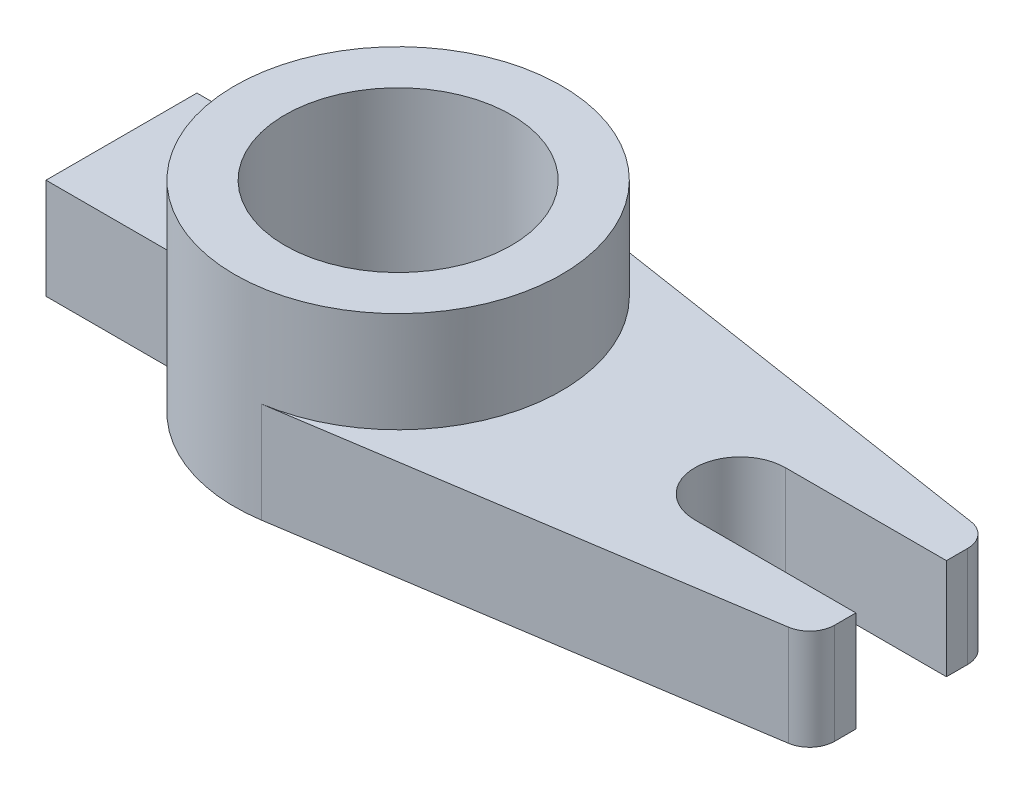
ISO-10303-21;
HEADER;
FILE_DESCRIPTION(('STEP AP214'),'2;1');
FILE_NAME('part.step','',(''),(''),'','','');
FILE_SCHEMA(('AUTOMOTIVE_DESIGN { 1 0 10303 214 1 1 1 1 }'));
ENDSEC;
DATA;
#1=APPLICATION_CONTEXT('core data for automotive mechanical design processes');
#2=APPLICATION_PROTOCOL_DEFINITION('international standard','automotive_design',2000,#1);
#3=PRODUCT_CONTEXT('',#1,'mechanical');
#4=PRODUCT('Part','Part','',(#3));
#5=PRODUCT_RELATED_PRODUCT_CATEGORY('part','',(#4));
#6=PRODUCT_DEFINITION_FORMATION('','',#4);
#7=PRODUCT_DEFINITION_CONTEXT('part definition',#1,'design');
#8=PRODUCT_DEFINITION('design','',#6,#7);
#9=PRODUCT_DEFINITION_SHAPE('','',#8);
#10=(LENGTH_UNIT() NAMED_UNIT(*) SI_UNIT(.MILLI.,.METRE.));
#11=(NAMED_UNIT(*) PLANE_ANGLE_UNIT() SI_UNIT($,.RADIAN.));
#12=(NAMED_UNIT(*) SI_UNIT($,.STERADIAN.) SOLID_ANGLE_UNIT());
#13=UNCERTAINTY_MEASURE_WITH_UNIT(LENGTH_MEASURE(1.E-05),#10,'distance_accuracy_value','');
#14=(GEOMETRIC_REPRESENTATION_CONTEXT(3) GLOBAL_UNCERTAINTY_ASSIGNED_CONTEXT((#13)) GLOBAL_UNIT_ASSIGNED_CONTEXT((#10,
#11,#12)) REPRESENTATION_CONTEXT('',''));
#15=CARTESIAN_POINT('',(0.,0.,0.));
#16=DIRECTION('',(0.,0.,1.));
#17=DIRECTION('',(1.,0.,0.));
#18=AXIS2_PLACEMENT_3D('',#15,#16,#17);
#19=CARTESIAN_POINT('',(0.,20.,0.));
#20=DIRECTION('',(0.,-1.,0.));
#21=DIRECTION('',(0.,0.,-1.));
#22=AXIS2_PLACEMENT_3D('',#19,#20,#21);
#23=CYLINDRICAL_SURFACE('',#22,32.5);
#24=CARTESIAN_POINT('',(0.,-20.,0.));
#25=DIRECTION('',(0.,1.,0.));
#26=DIRECTION('',(0.,0.,1.));
#27=AXIS2_PLACEMENT_3D('',#24,#25,#26);
#28=CIRCLE('',#27,32.5);
#29=CARTESIAN_POINT('',(4.94111598055763,-20.,-32.1221943968135));
#30=VERTEX_POINT('',#29);
#31=CARTESIAN_POINT('',(-28.831406486677,-20.,-15.));
#32=VERTEX_POINT('',#31);
#33=EDGE_CURVE('E45',#30,#32,#28,.T.);
#34=ORIENTED_EDGE('',*,*,#33,.T.);
#35=DIRECTION('',(0.,1.,0.));
#36=VECTOR('',#35,1.);
#37=CARTESIAN_POINT('',(-28.831406486677,-20.,-15.));
#38=LINE('',#37,#36);
#39=CARTESIAN_POINT('',(-28.831406486677,0.,-15.));
#40=VERTEX_POINT('',#39);
#41=EDGE_CURVE('E59',#32,#40,#38,.T.);
#42=ORIENTED_EDGE('',*,*,#41,.T.);
#43=CARTESIAN_POINT('',(0.,0.,0.));
#44=DIRECTION('',(0.,-1.,0.));
#45=DIRECTION('',(0.,0.,1.));
#46=AXIS2_PLACEMENT_3D('',#43,#44,#45);
#47=CIRCLE('',#46,32.5);
#48=CARTESIAN_POINT('',(-28.831406486677,0.,15.));
#49=VERTEX_POINT('',#48);
#50=EDGE_CURVE('E52',#49,#40,#47,.T.);
#51=ORIENTED_EDGE('',*,*,#50,.F.);
#52=DIRECTION('',(0.,1.,0.));
#53=VECTOR('',#52,1.);
#54=CARTESIAN_POINT('',(-28.831406486677,-20.,15.));
#55=LINE('',#54,#53);
#56=CARTESIAN_POINT('',(-28.831406486677,-20.,15.));
#57=VERTEX_POINT('',#56);
#58=EDGE_CURVE('E146',#57,#49,#55,.T.);
#59=ORIENTED_EDGE('',*,*,#58,.F.);
#60=CARTESIAN_POINT('',(4.94111598055763,-20.,32.1221943968135));
#61=VERTEX_POINT('',#60);
#62=EDGE_CURVE('E159',#57,#61,#28,.T.);
#63=ORIENTED_EDGE('',*,*,#62,.T.);
#64=DIRECTION('',(0.,1.,0.));
#65=VECTOR('',#64,1.);
#66=CARTESIAN_POINT('',(4.94111598055763,-20.,32.1221943968135));
#67=LINE('',#66,#65);
#68=CARTESIAN_POINT('',(4.94111598055763,0.,32.1221943968135));
#69=VERTEX_POINT('',#68);
#70=EDGE_CURVE('E236',#61,#69,#67,.T.);
#71=ORIENTED_EDGE('',*,*,#70,.T.);
#72=CARTESIAN_POINT('',(0.,0.,0.));
#73=DIRECTION('',(0.,-1.,0.));
#74=DIRECTION('',(0.,0.,1.));
#75=AXIS2_PLACEMENT_3D('',#72,#73,#74);
#76=CIRCLE('',#75,32.5);
#77=CARTESIAN_POINT('',(4.94111598055763,0.,-32.1221943968135));
#78=VERTEX_POINT('',#77);
#79=EDGE_CURVE('E227',#78,#69,#76,.T.);
#80=ORIENTED_EDGE('',*,*,#79,.F.);
#81=DIRECTION('',(0.,1.,0.));
#82=VECTOR('',#81,1.);
#83=CARTESIAN_POINT('',(4.94111598055763,-20.,-32.1221943968135));
#84=LINE('',#83,#82);
#85=EDGE_CURVE('E238',#30,#78,#84,.T.);
#86=ORIENTED_EDGE('',*,*,#85,.F.);
#87=EDGE_LOOP('',(#34,#42,#51,#59,#63,#71,#80,#86));
#88=FACE_BOUND('',#87,.T.);
#89=CARTESIAN_POINT('',(0.,20.,0.));
#90=DIRECTION('',(0.,1.,0.));
#91=DIRECTION('',(0.,0.,1.));
#92=AXIS2_PLACEMENT_3D('',#89,#90,#91);
#93=CIRCLE('',#92,32.5);
#94=CARTESIAN_POINT('',(0.,20.,32.5));
#95=VERTEX_POINT('',#94);
#96=EDGE_CURVE('E11',#95,#95,#93,.T.);
#97=ORIENTED_EDGE('',*,*,#96,.F.);
#98=EDGE_LOOP('',(#97));
#99=FACE_BOUND('',#98,.T.);
#100=ADVANCED_FACE('F39',(#88,#99),#23,.T.);
#101=CARTESIAN_POINT('',(0.,20.,0.));
#102=DIRECTION('',(0.,1.,0.));
#103=DIRECTION('',(0.,0.,1.));
#104=AXIS2_PLACEMENT_3D('',#101,#102,#103);
#105=PLANE('',#104);
#106=ORIENTED_EDGE('',*,*,#96,.T.);
#107=EDGE_LOOP('',(#106));
#108=FACE_BOUND('',#107,.T.);
#109=CARTESIAN_POINT('',(0.,20.,0.));
#110=DIRECTION('',(0.,1.,0.));
#111=DIRECTION('',(0.,0.,1.));
#112=AXIS2_PLACEMENT_3D('',#109,#110,#111);
#113=CIRCLE('',#112,22.5);
#114=CARTESIAN_POINT('',(0.,20.,22.5));
#115=VERTEX_POINT('',#114);
#116=EDGE_CURVE('E258',#115,#115,#113,.T.);
#117=ORIENTED_EDGE('',*,*,#116,.F.);
#118=EDGE_LOOP('',(#117));
#119=FACE_BOUND('',#118,.T.);
#120=ADVANCED_FACE('F274',(#108,#119),#105,.T.);
#121=CARTESIAN_POINT('',(0.,-20.,0.));
#122=DIRECTION('',(0.,1.,0.));
#123=DIRECTION('',(0.,0.,1.));
#124=AXIS2_PLACEMENT_3D('',#121,#122,#123);
#125=PLANE('',#124);
#126=ORIENTED_EDGE('',*,*,#33,.F.);
#127=DIRECTION('',(-0.988375212209647,0.,-0.152034337863312));
#128=VECTOR('',#127,1.);
#129=CARTESIAN_POINT('',(95.7601716893166,-20.,-18.1521809550725));
#130=LINE('',#129,#128);
#131=CARTESIAN_POINT('',(95.7601716893166,-20.,-18.1521809550726));
#132=VERTEX_POINT('',#131);
#133=EDGE_CURVE('E199',#132,#30,#130,.T.);
#134=ORIENTED_EDGE('',*,*,#133,.F.);
#135=CARTESIAN_POINT('',(95.,-20.,-13.2103048940244));
#136=DIRECTION('',(0.,1.,0.));
#137=DIRECTION('',(0.,0.,-1.));
#138=AXIS2_PLACEMENT_3D('',#135,#136,#137);
#139=CIRCLE('',#138,4.99999999999992);
#140=CARTESIAN_POINT('',(100.,-20.,-13.2103048940244));
#141=VERTEX_POINT('',#140);
#142=EDGE_CURVE('E197',#141,#132,#139,.T.);
#143=ORIENTED_EDGE('',*,*,#142,.F.);
#144=DIRECTION('',(0.,0.,-1.));
#145=VECTOR('',#144,1.);
#146=CARTESIAN_POINT('',(100.,-20.,-13.2103048940244));
#147=LINE('',#146,#145);
#148=CARTESIAN_POINT('',(100.,-20.,-9.));
#149=VERTEX_POINT('',#148);
#150=EDGE_CURVE('E193',#149,#141,#147,.T.);
#151=ORIENTED_EDGE('',*,*,#150,.F.);
#152=DIRECTION('',(1.,0.,0.));
#153=VECTOR('',#152,1.);
#154=CARTESIAN_POINT('',(100.,-20.,-9.));
#155=LINE('',#154,#153);
#156=CARTESIAN_POINT('',(68.,-20.,-9.));
#157=VERTEX_POINT('',#156);
#158=EDGE_CURVE('E194',#157,#149,#155,.T.);
#159=ORIENTED_EDGE('',*,*,#158,.F.);
#160=CARTESIAN_POINT('',(68.0000000000001,-20.,0.));
#161=DIRECTION('',(0.,-1.,0.));
#162=DIRECTION('',(0.,0.,1.));
#163=AXIS2_PLACEMENT_3D('',#160,#161,#162);
#164=CIRCLE('',#163,9.);
#165=CARTESIAN_POINT('',(68.,-20.,9.));
#166=VERTEX_POINT('',#165);
#167=EDGE_CURVE('E190',#166,#157,#164,.T.);
#168=ORIENTED_EDGE('',*,*,#167,.F.);
#169=DIRECTION('',(-1.,0.,0.));
#170=VECTOR('',#169,1.);
#171=CARTESIAN_POINT('',(68.,-20.,9.));
#172=LINE('',#171,#170);
#173=CARTESIAN_POINT('',(100.,-20.,9.));
#174=VERTEX_POINT('',#173);
#175=EDGE_CURVE('E183',#174,#166,#172,.T.);
#176=ORIENTED_EDGE('',*,*,#175,.F.);
#177=DIRECTION('',(0.,0.,-1.));
#178=VECTOR('',#177,1.);
#179=CARTESIAN_POINT('',(100.,-20.,9.));
#180=LINE('',#179,#178);
#181=CARTESIAN_POINT('',(100.,-20.,13.2103048940244));
#182=VERTEX_POINT('',#181);
#183=EDGE_CURVE('E182',#182,#174,#180,.T.);
#184=ORIENTED_EDGE('',*,*,#183,.F.);
#185=CARTESIAN_POINT('',(95.,-20.,13.2103048940244));
#186=DIRECTION('',(0.,1.,0.));
#187=DIRECTION('',(0.,0.,-1.));
#188=AXIS2_PLACEMENT_3D('',#185,#186,#187);
#189=CIRCLE('',#188,4.99999999999992);
#190=CARTESIAN_POINT('',(95.7601716893166,-20.,18.1521809550725));
#191=VERTEX_POINT('',#190);
#192=EDGE_CURVE('E180',#191,#182,#189,.T.);
#193=ORIENTED_EDGE('',*,*,#192,.F.);
#194=DIRECTION('',(0.988375212209647,0.,-0.152034337863312));
#195=VECTOR('',#194,1.);
#196=CARTESIAN_POINT('',(95.7601716893166,-20.,18.1521809550725));
#197=LINE('',#196,#195);
#198=EDGE_CURVE('E201',#61,#191,#197,.T.);
#199=ORIENTED_EDGE('',*,*,#198,.F.);
#200=ORIENTED_EDGE('',*,*,#62,.F.);
#201=DIRECTION('',(1.,0.,0.));
#202=VECTOR('',#201,1.);
#203=CARTESIAN_POINT('',(-55.,-20.,15.));
#204=LINE('',#203,#202);
#205=CARTESIAN_POINT('',(-55.,-20.,15.));
#206=VERTEX_POINT('',#205);
#207=EDGE_CURVE('E143',#206,#57,#204,.T.);
#208=ORIENTED_EDGE('',*,*,#207,.F.);
#209=DIRECTION('',(0.,0.,1.));
#210=VECTOR('',#209,1.);
#211=CARTESIAN_POINT('',(-55.,-20.,-15.));
#212=LINE('',#211,#210);
#213=CARTESIAN_POINT('',(-55.,-20.,-15.));
#214=VERTEX_POINT('',#213);
#215=EDGE_CURVE('E160',#214,#206,#212,.T.);
#216=ORIENTED_EDGE('',*,*,#215,.F.);
#217=DIRECTION('',(-1.,0.,0.));
#218=VECTOR('',#217,1.);
#219=CARTESIAN_POINT('',(-28.831406486677,-20.,-15.));
#220=LINE('',#219,#218);
#221=EDGE_CURVE('E149',#32,#214,#220,.T.);
#222=ORIENTED_EDGE('',*,*,#221,.F.);
#223=EDGE_LOOP('',(#126,#134,#143,#151,#159,#168,#176,#184,#193,#199,#200,#208,#216,#222));
#224=FACE_BOUND('',#223,.T.);
#225=CARTESIAN_POINT('',(0.,-20.,0.));
#226=DIRECTION('',(0.,1.,0.));
#227=DIRECTION('',(0.,0.,1.));
#228=AXIS2_PLACEMENT_3D('',#225,#226,#227);
#229=CIRCLE('',#228,22.5);
#230=CARTESIAN_POINT('',(0.,-20.,22.5));
#231=VERTEX_POINT('',#230);
#232=EDGE_CURVE('E240',#231,#231,#229,.T.);
#233=ORIENTED_EDGE('',*,*,#232,.T.);
#234=EDGE_LOOP('',(#233));
#235=FACE_BOUND('',#234,.T.);
#236=ADVANCED_FACE('F152',(#224,#235),#125,.F.);
#237=CARTESIAN_POINT('',(0.,20.,0.));
#238=DIRECTION('',(0.,-1.,0.));
#239=DIRECTION('',(0.,0.,-1.));
#240=AXIS2_PLACEMENT_3D('',#237,#238,#239);
#241=CYLINDRICAL_SURFACE('',#240,22.5);
#242=ORIENTED_EDGE('',*,*,#116,.T.);
#243=EDGE_LOOP('',(#242));
#244=FACE_BOUND('',#243,.T.);
#245=ORIENTED_EDGE('',*,*,#232,.F.);
#246=EDGE_LOOP('',(#245));
#247=FACE_BOUND('',#246,.T.);
#248=ADVANCED_FACE('F265',(#244,#247),#241,.F.);
#249=CARTESIAN_POINT('',(95.,-20.,13.2103048940244));
#250=DIRECTION('',(0.,1.,0.));
#251=DIRECTION('',(0.,0.,1.));
#252=AXIS2_PLACEMENT_3D('',#249,#250,#251);
#253=CYLINDRICAL_SURFACE('',#252,4.99999999999992);
#254=CARTESIAN_POINT('',(95.,0.,13.2103048940244));
#255=DIRECTION('',(0.,1.,0.));
#256=DIRECTION('',(0.,0.,-1.));
#257=AXIS2_PLACEMENT_3D('',#254,#255,#256);
#258=CIRCLE('',#257,4.99999999999992);
#259=CARTESIAN_POINT('',(95.7601716893166,0.,18.1521809550725));
#260=VERTEX_POINT('',#259);
#261=CARTESIAN_POINT('',(100.,0.,13.2103048940244));
#262=VERTEX_POINT('',#261);
#263=EDGE_CURVE('E172',#260,#262,#258,.T.);
#264=ORIENTED_EDGE('',*,*,#263,.F.);
#265=DIRECTION('',(0.,1.,0.));
#266=VECTOR('',#265,1.);
#267=CARTESIAN_POINT('',(95.7601716893166,-20.,18.1521809550725));
#268=LINE('',#267,#266);
#269=EDGE_CURVE('E232',#191,#260,#268,.T.);
#270=ORIENTED_EDGE('',*,*,#269,.F.);
#271=ORIENTED_EDGE('',*,*,#192,.T.);
#272=DIRECTION('',(0.,1.,0.));
#273=VECTOR('',#272,1.);
#274=CARTESIAN_POINT('',(100.,-20.,13.2103048940244));
#275=LINE('',#274,#273);
#276=EDGE_CURVE('E206',#182,#262,#275,.T.);
#277=ORIENTED_EDGE('',*,*,#276,.T.);
#278=EDGE_LOOP('',(#264,#270,#271,#277));
#279=FACE_BOUND('',#278,.T.);
#280=ADVANCED_FACE('F262',(#279),#253,.T.);
#281=CARTESIAN_POINT('',(95.7601716893166,-20.,18.1521809550725));
#282=DIRECTION('',(0.152034337863312,0.,0.988375212209647));
#283=DIRECTION('',(0.988375212209647,0.,-0.152034337863312));
#284=AXIS2_PLACEMENT_3D('',#281,#282,#283);
#285=PLANE('',#284);
#286=DIRECTION('',(0.988375212209647,0.,-0.152034337863312));
#287=VECTOR('',#286,1.);
#288=CARTESIAN_POINT('',(95.7601716893166,0.,18.1521809550725));
#289=LINE('',#288,#287);
#290=EDGE_CURVE('E185',#69,#260,#289,.T.);
#291=ORIENTED_EDGE('',*,*,#290,.F.);
#292=ORIENTED_EDGE('',*,*,#70,.F.);
#293=ORIENTED_EDGE('',*,*,#198,.T.);
#294=ORIENTED_EDGE('',*,*,#269,.T.);
#295=EDGE_LOOP('',(#291,#292,#293,#294));
#296=FACE_BOUND('',#295,.T.);
#297=ADVANCED_FACE('F271',(#296),#285,.T.);
#298=CARTESIAN_POINT('',(95.7601716893166,-20.,-18.1521809550725));
#299=DIRECTION('',(0.152034337863312,0.,-0.988375212209647));
#300=DIRECTION('',(-0.988375212209647,0.,-0.152034337863312));
#301=AXIS2_PLACEMENT_3D('',#298,#299,#300);
#302=PLANE('',#301);
#303=DIRECTION('',(-0.988375212209647,0.,-0.152034337863312));
#304=VECTOR('',#303,1.);
#305=CARTESIAN_POINT('',(95.7601716893166,0.,-18.1521809550725));
#306=LINE('',#305,#304);
#307=CARTESIAN_POINT('',(95.7601716893166,0.,-18.1521809550726));
#308=VERTEX_POINT('',#307);
#309=EDGE_CURVE('E226',#308,#78,#306,.T.);
#310=ORIENTED_EDGE('',*,*,#309,.F.);
#311=DIRECTION('',(0.,1.,0.));
#312=VECTOR('',#311,1.);
#313=CARTESIAN_POINT('',(95.7601716893166,-20.,-18.1521809550726));
#314=LINE('',#313,#312);
#315=EDGE_CURVE('E245',#132,#308,#314,.T.);
#316=ORIENTED_EDGE('',*,*,#315,.F.);
#317=ORIENTED_EDGE('',*,*,#133,.T.);
#318=ORIENTED_EDGE('',*,*,#85,.T.);
#319=EDGE_LOOP('',(#310,#316,#317,#318));
#320=FACE_BOUND('',#319,.T.);
#321=ADVANCED_FACE('F310',(#320),#302,.T.);
#322=CARTESIAN_POINT('',(95.,-20.,-13.2103048940244));
#323=DIRECTION('',(0.,1.,0.));
#324=DIRECTION('',(0.,0.,1.));
#325=AXIS2_PLACEMENT_3D('',#322,#323,#324);
#326=CYLINDRICAL_SURFACE('',#325,4.99999999999992);
#327=CARTESIAN_POINT('',(95.,0.,-13.2103048940244));
#328=DIRECTION('',(0.,1.,0.));
#329=DIRECTION('',(0.,0.,-1.));
#330=AXIS2_PLACEMENT_3D('',#327,#328,#329);
#331=CIRCLE('',#330,4.99999999999992);
#332=CARTESIAN_POINT('',(100.,0.,-13.2103048940244));
#333=VERTEX_POINT('',#332);
#334=EDGE_CURVE('E221',#333,#308,#331,.T.);
#335=ORIENTED_EDGE('',*,*,#334,.F.);
#336=DIRECTION('',(0.,1.,0.));
#337=VECTOR('',#336,1.);
#338=CARTESIAN_POINT('',(100.,-20.,-13.2103048940244));
#339=LINE('',#338,#337);
#340=EDGE_CURVE('E242',#141,#333,#339,.T.);
#341=ORIENTED_EDGE('',*,*,#340,.F.);
#342=ORIENTED_EDGE('',*,*,#142,.T.);
#343=ORIENTED_EDGE('',*,*,#315,.T.);
#344=EDGE_LOOP('',(#335,#341,#342,#343));
#345=FACE_BOUND('',#344,.T.);
#346=ADVANCED_FACE('F311',(#345),#326,.T.);
#347=CARTESIAN_POINT('',(100.,-20.,-13.2103048940244));
#348=DIRECTION('',(1.,0.,0.));
#349=DIRECTION('',(0.,0.,-1.));
#350=AXIS2_PLACEMENT_3D('',#347,#348,#349);
#351=PLANE('',#350);
#352=DIRECTION('',(0.,0.,-1.));
#353=VECTOR('',#352,1.);
#354=CARTESIAN_POINT('',(100.,0.,-13.2103048940244));
#355=LINE('',#354,#353);
#356=CARTESIAN_POINT('',(100.,0.,-9.));
#357=VERTEX_POINT('',#356);
#358=EDGE_CURVE('E222',#357,#333,#355,.T.);
#359=ORIENTED_EDGE('',*,*,#358,.F.);
#360=DIRECTION('',(0.,1.,0.));
#361=VECTOR('',#360,1.);
#362=CARTESIAN_POINT('',(100.,-20.,-9.));
#363=LINE('',#362,#361);
#364=EDGE_CURVE('E246',#149,#357,#363,.T.);
#365=ORIENTED_EDGE('',*,*,#364,.F.);
#366=ORIENTED_EDGE('',*,*,#150,.T.);
#367=ORIENTED_EDGE('',*,*,#340,.T.);
#368=EDGE_LOOP('',(#359,#365,#366,#367));
#369=FACE_BOUND('',#368,.T.);
#370=ADVANCED_FACE('F320',(#369),#351,.T.);
#371=CARTESIAN_POINT('',(100.,-20.,-9.));
#372=DIRECTION('',(0.,0.,1.));
#373=DIRECTION('',(1.,0.,0.));
#374=AXIS2_PLACEMENT_3D('',#371,#372,#373);
#375=PLANE('',#374);
#376=DIRECTION('',(1.,0.,0.));
#377=VECTOR('',#376,1.);
#378=CARTESIAN_POINT('',(100.,0.,-9.));
#379=LINE('',#378,#377);
#380=CARTESIAN_POINT('',(68.,0.,-9.));
#381=VERTEX_POINT('',#380);
#382=EDGE_CURVE('E217',#381,#357,#379,.T.);
#383=ORIENTED_EDGE('',*,*,#382,.F.);
#384=DIRECTION('',(0.,1.,0.));
#385=VECTOR('',#384,1.);
#386=CARTESIAN_POINT('',(68.,-20.,-9.));
#387=LINE('',#386,#385);
#388=EDGE_CURVE('E248',#157,#381,#387,.T.);
#389=ORIENTED_EDGE('',*,*,#388,.F.);
#390=ORIENTED_EDGE('',*,*,#158,.T.);
#391=ORIENTED_EDGE('',*,*,#364,.T.);
#392=EDGE_LOOP('',(#383,#389,#390,#391));
#393=FACE_BOUND('',#392,.T.);
#394=ADVANCED_FACE('F321',(#393),#375,.T.);
#395=CARTESIAN_POINT('',(68.0000000000001,-20.,0.));
#396=DIRECTION('',(0.,1.,0.));
#397=DIRECTION('',(0.,0.,1.));
#398=AXIS2_PLACEMENT_3D('',#395,#396,#397);
#399=CYLINDRICAL_SURFACE('',#398,9.);
#400=CARTESIAN_POINT('',(68.0000000000001,0.,0.));
#401=DIRECTION('',(0.,-1.,0.));
#402=DIRECTION('',(0.,0.,1.));
#403=AXIS2_PLACEMENT_3D('',#400,#401,#402);
#404=CIRCLE('',#403,9.);
#405=CARTESIAN_POINT('',(68.,0.,9.));
#406=VERTEX_POINT('',#405);
#407=EDGE_CURVE('E214',#406,#381,#404,.T.);
#408=ORIENTED_EDGE('',*,*,#407,.F.);
#409=DIRECTION('',(0.,1.,0.));
#410=VECTOR('',#409,1.);
#411=CARTESIAN_POINT('',(68.,-20.,9.));
#412=LINE('',#411,#410);
#413=EDGE_CURVE('E253',#166,#406,#412,.T.);
#414=ORIENTED_EDGE('',*,*,#413,.F.);
#415=ORIENTED_EDGE('',*,*,#167,.T.);
#416=ORIENTED_EDGE('',*,*,#388,.T.);
#417=EDGE_LOOP('',(#408,#414,#415,#416));
#418=FACE_BOUND('',#417,.T.);
#419=ADVANCED_FACE('F324',(#418),#399,.F.);
#420=CARTESIAN_POINT('',(68.,-20.,9.));
#421=DIRECTION('',(0.,0.,-1.));
#422=DIRECTION('',(-1.,0.,0.));
#423=AXIS2_PLACEMENT_3D('',#420,#421,#422);
#424=PLANE('',#423);
#425=DIRECTION('',(-1.,0.,0.));
#426=VECTOR('',#425,1.);
#427=CARTESIAN_POINT('',(68.,0.,9.));
#428=LINE('',#427,#426);
#429=CARTESIAN_POINT('',(100.,0.,9.));
#430=VERTEX_POINT('',#429);
#431=EDGE_CURVE('E215',#430,#406,#428,.T.);
#432=ORIENTED_EDGE('',*,*,#431,.F.);
#433=DIRECTION('',(0.,1.,0.));
#434=VECTOR('',#433,1.);
#435=CARTESIAN_POINT('',(100.,-20.,9.));
#436=LINE('',#435,#434);
#437=EDGE_CURVE('E251',#174,#430,#436,.T.);
#438=ORIENTED_EDGE('',*,*,#437,.F.);
#439=ORIENTED_EDGE('',*,*,#175,.T.);
#440=ORIENTED_EDGE('',*,*,#413,.T.);
#441=EDGE_LOOP('',(#432,#438,#439,#440));
#442=FACE_BOUND('',#441,.T.);
#443=ADVANCED_FACE('F328',(#442),#424,.T.);
#444=CARTESIAN_POINT('',(100.,-20.,9.));
#445=DIRECTION('',(1.,0.,0.));
#446=DIRECTION('',(0.,0.,-1.));
#447=AXIS2_PLACEMENT_3D('',#444,#445,#446);
#448=PLANE('',#447);
#449=DIRECTION('',(0.,0.,-1.));
#450=VECTOR('',#449,1.);
#451=CARTESIAN_POINT('',(100.,0.,9.));
#452=LINE('',#451,#450);
#453=EDGE_CURVE('E207',#262,#430,#452,.T.);
#454=ORIENTED_EDGE('',*,*,#453,.F.);
#455=ORIENTED_EDGE('',*,*,#276,.F.);
#456=ORIENTED_EDGE('',*,*,#183,.T.);
#457=ORIENTED_EDGE('',*,*,#437,.T.);
#458=EDGE_LOOP('',(#454,#455,#456,#457));
#459=FACE_BOUND('',#458,.T.);
#460=ADVANCED_FACE('F302',(#459),#448,.T.);
#461=CARTESIAN_POINT('',(95.,0.,13.2103048940244));
#462=DIRECTION('',(0.,-1.,0.));
#463=DIRECTION('',(0.,0.,-1.));
#464=AXIS2_PLACEMENT_3D('',#461,#462,#463);
#465=PLANE('',#464);
#466=ORIENTED_EDGE('',*,*,#263,.T.);
#467=ORIENTED_EDGE('',*,*,#453,.T.);
#468=ORIENTED_EDGE('',*,*,#431,.T.);
#469=ORIENTED_EDGE('',*,*,#407,.T.);
#470=ORIENTED_EDGE('',*,*,#382,.T.);
#471=ORIENTED_EDGE('',*,*,#358,.T.);
#472=ORIENTED_EDGE('',*,*,#334,.T.);
#473=ORIENTED_EDGE('',*,*,#309,.T.);
#474=ORIENTED_EDGE('',*,*,#79,.T.);
#475=ORIENTED_EDGE('',*,*,#290,.T.);
#476=EDGE_LOOP('',(#466,#467,#468,#469,#470,#471,#472,#473,#474,#475));
#477=FACE_BOUND('',#476,.T.);
#478=ADVANCED_FACE('F305',(#477),#465,.F.);
#479=CARTESIAN_POINT('',(-55.,-20.,-15.));
#480=DIRECTION('',(-1.,0.,0.));
#481=DIRECTION('',(0.,0.,1.));
#482=AXIS2_PLACEMENT_3D('',#479,#480,#481);
#483=PLANE('',#482);
#484=DIRECTION('',(0.,0.,1.));
#485=VECTOR('',#484,1.);
#486=CARTESIAN_POINT('',(-55.,0.,-15.));
#487=LINE('',#486,#485);
#488=CARTESIAN_POINT('',(-55.,0.,-15.));
#489=VERTEX_POINT('',#488);
#490=CARTESIAN_POINT('',(-55.,0.,15.));
#491=VERTEX_POINT('',#490);
#492=EDGE_CURVE('E168',#489,#491,#487,.T.);
#493=ORIENTED_EDGE('',*,*,#492,.F.);
#494=DIRECTION('',(0.,1.,0.));
#495=VECTOR('',#494,1.);
#496=CARTESIAN_POINT('',(-55.,-20.,-15.));
#497=LINE('',#496,#495);
#498=EDGE_CURVE('E162',#214,#489,#497,.T.);
#499=ORIENTED_EDGE('',*,*,#498,.F.);
#500=ORIENTED_EDGE('',*,*,#215,.T.);
#501=DIRECTION('',(0.,1.,0.));
#502=VECTOR('',#501,1.);
#503=CARTESIAN_POINT('',(-55.,-20.,15.));
#504=LINE('',#503,#502);
#505=EDGE_CURVE('E140',#206,#491,#504,.T.);
#506=ORIENTED_EDGE('',*,*,#505,.T.);
#507=EDGE_LOOP('',(#493,#499,#500,#506));
#508=FACE_BOUND('',#507,.T.);
#509=ADVANCED_FACE('F165',(#508),#483,.T.);
#510=CARTESIAN_POINT('',(-28.831406486677,-20.,-15.));
#511=DIRECTION('',(0.,0.,-1.));
#512=DIRECTION('',(-1.,0.,0.));
#513=AXIS2_PLACEMENT_3D('',#510,#511,#512);
#514=PLANE('',#513);
#515=DIRECTION('',(-1.,0.,0.));
#516=VECTOR('',#515,1.);
#517=CARTESIAN_POINT('',(-28.831406486677,0.,-15.));
#518=LINE('',#517,#516);
#519=EDGE_CURVE('E163',#40,#489,#518,.T.);
#520=ORIENTED_EDGE('',*,*,#519,.F.);
#521=ORIENTED_EDGE('',*,*,#41,.F.);
#522=ORIENTED_EDGE('',*,*,#221,.T.);
#523=ORIENTED_EDGE('',*,*,#498,.T.);
#524=EDGE_LOOP('',(#520,#521,#522,#523));
#525=FACE_BOUND('',#524,.T.);
#526=ADVANCED_FACE('F288',(#525),#514,.T.);
#527=CARTESIAN_POINT('',(-55.,-20.,15.));
#528=DIRECTION('',(0.,0.,1.));
#529=DIRECTION('',(1.,0.,0.));
#530=AXIS2_PLACEMENT_3D('',#527,#528,#529);
#531=PLANE('',#530);
#532=DIRECTION('',(1.,0.,0.));
#533=VECTOR('',#532,1.);
#534=CARTESIAN_POINT('',(-55.,0.,15.));
#535=LINE('',#534,#533);
#536=EDGE_CURVE('E141',#491,#49,#535,.T.);
#537=ORIENTED_EDGE('',*,*,#536,.F.);
#538=ORIENTED_EDGE('',*,*,#505,.F.);
#539=ORIENTED_EDGE('',*,*,#207,.T.);
#540=ORIENTED_EDGE('',*,*,#58,.T.);
#541=EDGE_LOOP('',(#537,#538,#539,#540));
#542=FACE_BOUND('',#541,.T.);
#543=ADVANCED_FACE('F137',(#542),#531,.T.);
#544=CARTESIAN_POINT('',(0.,0.,0.));
#545=DIRECTION('',(0.,1.,0.));
#546=DIRECTION('',(0.,0.,1.));
#547=AXIS2_PLACEMENT_3D('',#544,#545,#546);
#548=PLANE('',#547);
#549=ORIENTED_EDGE('',*,*,#492,.T.);
#550=ORIENTED_EDGE('',*,*,#536,.T.);
#551=ORIENTED_EDGE('',*,*,#50,.T.);
#552=ORIENTED_EDGE('',*,*,#519,.T.);
#553=EDGE_LOOP('',(#549,#550,#551,#552));
#554=FACE_BOUND('',#553,.T.);
#555=ADVANCED_FACE('F292',(#554),#548,.T.);
#556=CLOSED_SHELL('',(#100,#120,#236,#248,#280,#297,#321,#346,#370,#394,#419,#443,#460,#478,
#509,#526,#543,#555));
#557=MANIFOLD_SOLID_BREP('B2',#556);
#558=ADVANCED_BREP_SHAPE_REPRESENTATION('',(#18,#557),#14);
#559=SHAPE_DEFINITION_REPRESENTATION(#9,#558);
ENDSEC;
END-ISO-10303-21;
